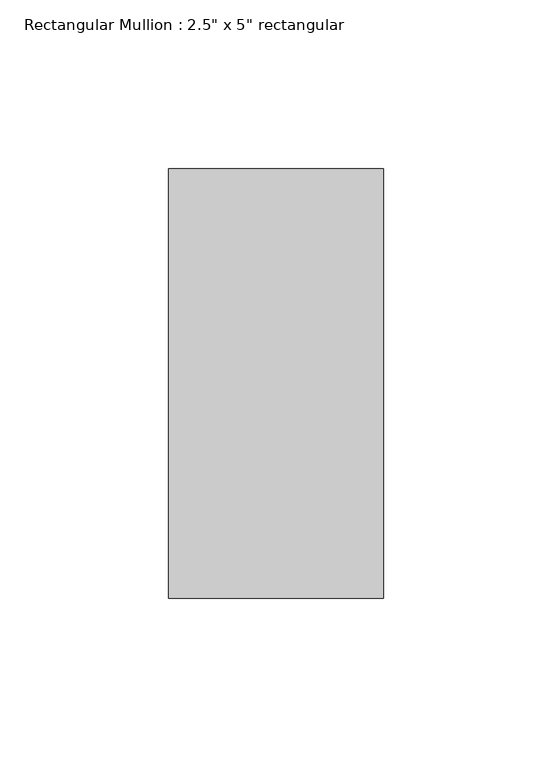
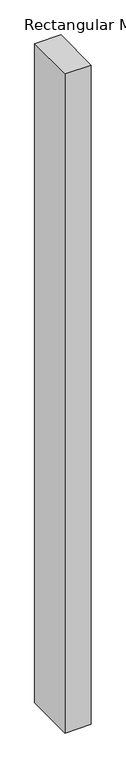
"""IFC4 building model written with IfcOpenShell, lengths in millimetres: member geometry."""

from ifc_helpers import new_model, si_unit, frame, origin, place, context, project, spatial, polyline, outline, extrude, source, transform, mapped, element, save


def member_637ca32e(model_context):
    return source(origin(), model_context, "Body", "SweptSolid", [
        extrude(outline(polyline([(0.0, 63.5), (0.0, -63.5), (-63.5, -63.5), (-63.5, 63.5), (0.0, 63.5)])), frame((0.0, 0.0, -1686.2136257), z_axis=(0.0, 0.0, 1.0), x_axis=(1.0, 0.0, 0.0)), (0.0, 0.0, 1.0), 1686.2136257),
    ])


if __name__ == "__main__":
    model = new_model("IFC4")
    model_context = context("Model", 3, world=origin())
    ifc_project = project(units=[si_unit("LENGTHUNIT", "METRE", prefix="MILLI")], contexts=[model_context])
    site = spatial("IfcSite", under=ifc_project)
    building = spatial("IfcBuilding", under=site)
    placement = place(None, origin())
    member_shape = member_637ca32e(model_context)
    element("IfcMember", 1, ObjectType="Rectangular Mullion : 2.5\" x 5\" rectangular", at=placement, inside=building, context=model_context, shape_type="MappedRepresentation", body=[
        mapped(member_shape, transform((0.0, 0.0, 0.0), x_axis=(1.0, 0.0, 0.0), y_axis=(0.0, 1.0, 0.0), z_axis=(0.0, 0.0, 1.0))),
    ])
    save(model, "model.ifc")

# Revit data of these elements
# Type "Rectangular Mullion : 2.5\" x 5\" rectangular"
#   built-in parameter 1007304 = 0.416667 (stored number, unit not read)
#   built-in parameter 1007301 = 0.104167 (stored number, unit not read)
#   built-in parameter 1007300 = 0.104167 (stored number, unit not read)
# Element 1 (IfcMember, "Rectangular Mullion : 2.5\" x 5\" rectangular")
#   Materials on its faces: "Aluminum"
# Materials
#   "Aluminum": class "Metal", colour RGB 247 247 247, transparency 0, Description = "Aluminum 6061", Cost = 0
